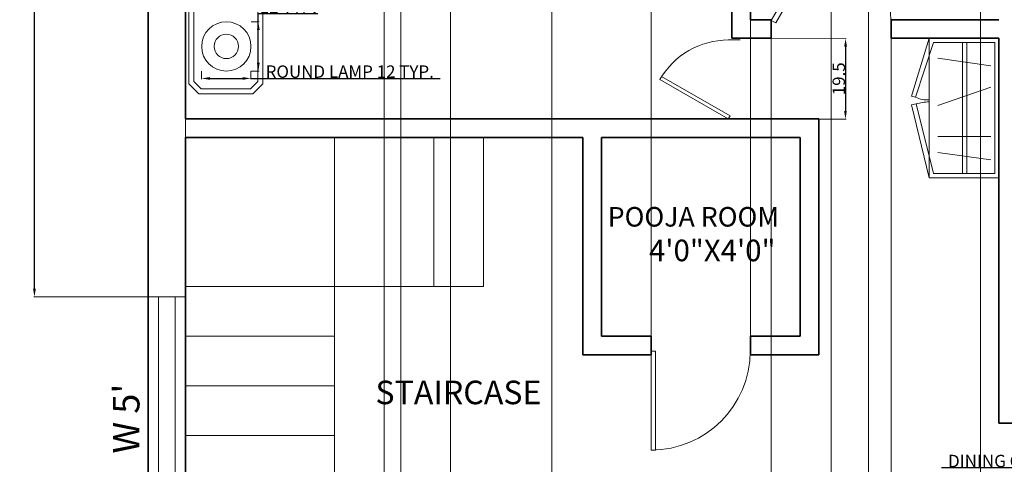
# Model space of a CAD drawing. Units: feet. Extents: x -297 to 770, y -228 to 625.
# Tile 6 of 14: x 351 to 589, y 95 to 202. Entities that reach past the tile are written whole.
import ezdxf

# ---------------------------------------------------------------- set-up
doc = ezdxf.new("R2010")
doc.units = ezdxf.units.FT
doc.header["$MEASUREMENT"] = 0
for name, color, linetype, lineweight in [('A-ANNO-DIMS', 2, 'Continuous', 18), ('A-ANNO-TEXT', 7, 'Continuous', 18), ('A-AREA-IDEN', 7, 'Continuous', 25), ('A-FLOR-STRS', 7, 'Continuous', 18), ('A-FURN', 8, 'Continuous', 18), ('A-WALL', 7, 'Continuous', 35), ('doors', 30, 'Continuous', 18), ('windows', 30, 'Continuous', 18)]:
    doc.layers.add(name, color=color, linetype=linetype, lineweight=lineweight)
doc.styles.add('Annotative', font='arial.ttf')
doc.styles.get("Standard").update_dxf_attribs({"font": 'arial.ttf'})
doc.dimstyles.get("Standard").update_dxf_attribs({"dimtxt": 3, "dimasz": 2, "dimexe": 0.18, "dimexo": 0.0625, "dimgap": 0.09, "dimtad": 1, "dimtoh": 1, "dimdec": 1, "dimzin": 0, "dimdsep": 46, "dimlunit": 3, "dimtxsty": 'Standard', "dimcen": 0, "dimclre": 256, "dimadec": 0, "dimazin": 0, "dimtfac": 1, "dimtdec": 1, "dimtofl": 0, "dimtmove": 0, "dimatfit": 3, "dimfxl": 1, "dimtolj": 1, "dimtzin": 0, "dimlwe": -1, "dimarcsym": 0})

# ---------------------------------------------------------------- blocks, each defined once
blk = doc.blocks.new('*U3')
for p, q in [((0, 0), (0, -6)), ((40, 0), (40, -6))]:
    blk.add_line(p, q)
blk.add_lwpolyline([(0, 0), (20, 34.64), (21.52, 33.77), (1.52, -0.88)], close=True)
blk.add_arc((0, 0), 40, 0, 60)
blk = doc.blocks.new('*U4')
for p, q in [((0, 0), (0, 6)), ((40, 0), (40, 6))]:
    blk.add_line(p, q)
blk.add_lwpolyline([(0, 0), (0, -40), (1.75, -40), (1.75, 0)], close=True)
blk.add_arc((0, 0), 40, 270, 0)
blk = doc.blocks.new('WIN-5FT')
for p, q in [((60, 6.5), (0, 6.5)), ((60, 2.5), (0, 2.5))]:
    blk.add_line(p, q)
blk.add_lwpolyline([(60, 0), (60, 9), (0, 9), (0, 0)], close=True)
blk = doc.blocks.new('LAMP-BEDSIDE-ROUND')
for radius in [5.95, 2.95]:
    blk.add_circle((5.95, 5.95), radius)
blk = doc.blocks.new('NIGHTSTAND')
for points in [[(17.84, 2.38), (17.84, 21.41), (15.46, 23.79), (2.38, 23.79), (0, 21.41), (0, 2.38), (2.38, 0), (15.46, 0)], [(16.65, 2.97), (16.65, 20.81), (14.87, 22.6), (2.97, 22.6), (1.19, 20.81), (1.19, 2.97), (2.97, 1.19), (14.87, 1.19)]]:
    blk.add_lwpolyline(points, close=True)
blk = doc.blocks.new('*D23')
at = {"layer": 'A-ANNO-DIMS', "color": 0, "lineweight": -2, "transparency": 16777216}
for p, q in [((620.45, 93.67), (573.78, 93.67)), ((631.66, 93.67), (622.45, 93.67))]:
    blk.add_line(p, q, dxfattribs=at)
at = {"layer": 'A-ANNO-DIMS', "transparency": 16777216}
for p, q in [((620.45, 91.75), (620.45, 93.85)), ((633.66, 91.75), (633.66, 93.85))]:
    blk.add_line(p, q, dxfattribs=at)
at = {"layer": 'A-ANNO-DIMS', "color": 0, "transparency": 16777216}
for points in [[(622.45, 94), (622.45, 93.33), (620.45, 93.67)], [(631.66, 94), (631.66, 93.33), (633.66, 93.67)]]:
    blk.add_solid(points, dxfattribs=at)
at = {"layer": 'Defpoints', "color": 0, "transparency": 16777216}
for p in [(620.45, 93.67), (620.45, 91.69), (633.66, 91.69)]:
    blk.add_point(p, dxfattribs=at)
at = {"layer": 'A-ANNO-DIMS', "color": 0, "transparency": 16777216, "insert": (596.11, 95.31), "char_height": 3, "attachment_point": 5}
blk.add_mtext('\\A1;DINING CHAIR 13 TYP.', dxfattribs=at)
blk = doc.blocks.new('*D27')
at = {"layer": 'A-ANNO-DIMS', "transparency": 16777216}
for p, q in [((395.09, 189.49), (395.09, 187.59)), ((406.99, 189.49), (406.99, 187.59))]:
    blk.add_line(p, q, dxfattribs=at)
at = {"layer": 'A-ANNO-DIMS', "color": 0, "lineweight": -2, "transparency": 16777216}
for p, q in [((397.09, 187.77), (404.99, 187.77)), ((406.99, 187.77), (452.72, 187.77))]:
    blk.add_line(p, q, dxfattribs=at)
at = {"layer": 'A-ANNO-DIMS', "color": 0, "transparency": 16777216}
for points in [[(397.09, 188.1), (397.09, 187.43), (395.09, 187.77)], [(404.99, 188.1), (404.99, 187.43), (406.99, 187.77)]]:
    blk.add_solid(points, dxfattribs=at)
at = {"layer": 'Defpoints', "color": 0, "transparency": 16777216}
for p in [(395.09, 189.55), (406.99, 189.55), (406.99, 187.77)]:
    blk.add_point(p, dxfattribs=at)
at = {"layer": 'A-ANNO-DIMS', "color": 0, "transparency": 16777216, "insert": (430.86, 189.41), "char_height": 3, "attachment_point": 5}
blk.add_mtext('\\A1;ROUND LAMP 12 TYP.', dxfattribs=at)
blk = doc.blocks.new('*D28')
at = {"layer": 'A-ANNO-DIMS', "color": 0, "lineweight": -2, "transparency": 16777216}
for p, q in [((408.77, 201.45), (408.77, 203.45)), ((408.77, 203.45), (423.18, 203.45)), ((408.77, 191.55), (408.77, 199.45))]:
    blk.add_line(p, q, dxfattribs=at)
at = {"layer": 'A-ANNO-DIMS', "transparency": 16777216}
for p, q in [((407.05, 201.45), (408.95, 201.45)), ((407.05, 189.55), (408.95, 189.55))]:
    blk.add_line(p, q, dxfattribs=at)
at = {"layer": 'A-ANNO-DIMS', "color": 0, "transparency": 16777216}
for points in [[(408.44, 199.45), (409.11, 199.45), (408.77, 201.45)], [(408.44, 191.55), (409.11, 191.55), (408.77, 189.55)]]:
    blk.add_solid(points, dxfattribs=at)
at = {"layer": 'Defpoints', "color": 0, "transparency": 16777216}
for p in [(406.99, 201.45), (408.77, 201.45), (406.99, 189.55)]:
    blk.add_point(p, dxfattribs=at)
at = {"layer": 'A-ANNO-DIMS', "color": 0, "transparency": 16777216, "insert": (416.02, 205.04), "char_height": 3, "attachment_point": 5}
blk.add_mtext('\\A1;12 TYP.', dxfattribs=at)
blk = doc.blocks.new('*D51')
at = {"layer": 'A-ANNO-DIMS', "transparency": 16777216}
for p, q in [((382.09, 306.96), (354.53, 306.96)), ((382.09, 134.96), (354.53, 134.96))]:
    blk.add_line(p, q, dxfattribs=at)
at = {"layer": 'A-ANNO-DIMS', "color": 0, "lineweight": -2, "transparency": 16777216}
blk.add_line((354.71, 136.96), (354.71, 304.96), dxfattribs=at)
at = {"layer": 'A-ANNO-DIMS', "color": 0, "transparency": 16777216}
for points in [[(354.37, 304.96), (355.04, 304.96), (354.71, 306.96)], [(354.37, 136.96), (355.04, 136.96), (354.71, 134.96)]]:
    blk.add_solid(points, dxfattribs=at)
at = {"layer": 'Defpoints', "color": 0, "transparency": 16777216}
for p in [(354.71, 306.96), (382.16, 306.96), (382.16, 134.96)]:
    blk.add_point(p, dxfattribs=at)
at = {"layer": 'A-ANNO-DIMS', "color": 0, "transparency": 16777216, "insert": (353.11, 220.96), "char_height": 3, "attachment_point": 5, "rotation": 90}
blk.add_mtext('\\A1;172', dxfattribs=at)
blk = doc.blocks.new('*D57')
at = {"layer": 'A-ANNO-DIMS', "transparency": 16777216}
for p, q in [((391.16, -163.97), (391.16, 367.22)), ((439.16, -163.97), (439.16, 367.22))]:
    blk.add_line(p, q, dxfattribs=at)
at = {"layer": 'A-ANNO-DIMS', "color": 0, "lineweight": -2, "transparency": 16777216}
blk.add_line((393.16, 367.04), (437.16, 367.04), dxfattribs=at)
at = {"layer": 'A-ANNO-DIMS', "color": 0, "transparency": 16777216}
for points in [[(393.16, 367.38), (393.16, 366.71), (391.16, 367.04)], [(437.16, 367.38), (437.16, 366.71), (439.16, 367.04)]]:
    blk.add_solid(points, dxfattribs=at)
at = {"layer": 'Defpoints', "color": 0, "transparency": 16777216}
for p in [(439.16, 367.04), (391.16, -164.04), (439.16, -164.04)]:
    blk.add_point(p, dxfattribs=at)
at = {"layer": 'A-ANNO-DIMS', "color": 0, "transparency": 16777216, "insert": (415.16, 368.66), "char_height": 3, "attachment_point": 5}
blk.add_mtext('\\A1;48', dxfattribs=at)
blk = doc.blocks.new('*D60')
at = {"layer": 'A-ANNO-DIMS', "transparency": 16777216}
for p, q in [((556.16, -144.47), (556.16, 367.22)), ((583.16, -144.47), (583.16, 367.22))]:
    blk.add_line(p, q, dxfattribs=at)
at = {"layer": 'A-ANNO-DIMS', "color": 0, "lineweight": -2, "transparency": 16777216}
blk.add_line((558.16, 367.04), (581.16, 367.04), dxfattribs=at)
at = {"layer": 'A-ANNO-DIMS', "color": 0, "transparency": 16777216}
for points in [[(558.16, 367.38), (558.16, 366.71), (556.16, 367.04)], [(581.16, 367.38), (581.16, 366.71), (583.16, 367.04)]]:
    blk.add_solid(points, dxfattribs=at)
at = {"layer": 'Defpoints', "color": 0, "transparency": 16777216}
for p in [(583.16, 367.04), (556.16, -144.54), (583.16, -144.54)]:
    blk.add_point(p, dxfattribs=at)
at = {"layer": 'A-ANNO-DIMS', "color": 0, "transparency": 16777216, "insert": (569.66, 368.64), "char_height": 3, "attachment_point": 5}
blk.add_mtext('\\A1;27', dxfattribs=at)
blk = doc.blocks.new('*D66')
at = {"layer": 'A-ANNO-DIMS', "transparency": 16777216}
for p, q in [((503.66, 125.53), (503.66, 367.22)), ((527.66, 125.53), (527.66, 367.22))]:
    blk.add_line(p, q, dxfattribs=at)
at = {"layer": 'A-ANNO-DIMS', "color": 0, "lineweight": -2, "transparency": 16777216}
blk.add_line((505.66, 367.04), (525.66, 367.04), dxfattribs=at)
at = {"layer": 'A-ANNO-DIMS', "color": 0, "transparency": 16777216}
for points in [[(505.66, 367.38), (505.66, 366.71), (503.66, 367.04)], [(525.66, 367.38), (525.66, 366.71), (527.66, 367.04)]]:
    blk.add_solid(points, dxfattribs=at)
at = {"layer": 'Defpoints', "color": 0, "transparency": 16777216}
for p in [(527.66, 367.04), (503.66, 125.46), (527.66, 125.46)]:
    blk.add_point(p, dxfattribs=at)
at = {"layer": 'A-ANNO-DIMS', "color": 0, "transparency": 16777216, "insert": (515.66, 368.64), "char_height": 3, "attachment_point": 5}
blk.add_mtext('\\A1;24', dxfattribs=at)
blk = doc.blocks.new('*D67')
at = {"layer": 'A-ANNO-DIMS', "transparency": 16777216}
for p, q in [((532.66, 197.4), (532.66, -227.67)), ((561.66, 197.4), (561.66, -227.67))]:
    blk.add_line(p, q, dxfattribs=at)
at = {"layer": 'A-ANNO-DIMS', "color": 0, "lineweight": -2, "transparency": 16777216}
blk.add_line((534.66, -227.49), (559.66, -227.49), dxfattribs=at)
at = {"layer": 'A-ANNO-DIMS', "color": 0, "transparency": 16777216}
for points in [[(534.66, -227.15), (534.66, -227.82), (532.66, -227.49)], [(559.66, -227.15), (559.66, -227.82), (561.66, -227.49)]]:
    blk.add_solid(points, dxfattribs=at)
at = {"layer": 'Defpoints', "color": 0, "transparency": 16777216}
for p in [(532.66, 197.46), (561.66, 197.46), (561.66, -227.49)]:
    blk.add_point(p, dxfattribs=at)
at = {"layer": 'A-ANNO-DIMS', "color": 0, "transparency": 16777216, "insert": (547.16, -225.87), "char_height": 3, "attachment_point": 5}
blk.add_mtext('\\A1;29', dxfattribs=at)
blk = doc.blocks.new('*D71')
at = {"layer": 'A-ANNO-DIMS', "transparency": 16777216}
for p, q in [((523.22, 197.46), (550.79, 197.42)), ((523.19, 177.96), (550.76, 177.92))]:
    blk.add_line(p, q, dxfattribs=at)
at = {"layer": 'A-ANNO-DIMS', "color": 0, "lineweight": -2, "transparency": 16777216}
blk.add_line((550.6, 195.42), (550.58, 179.92), dxfattribs=at)
at = {"layer": 'A-ANNO-DIMS', "color": 0, "transparency": 16777216}
for points in [[(550.27, 195.42), (550.94, 195.42), (550.61, 197.42)], [(550.25, 179.92), (550.91, 179.92), (550.58, 177.92)]]:
    blk.add_solid(points, dxfattribs=at)
at = {"layer": 'Defpoints', "color": 0, "transparency": 16777216}
for p in [(523.16, 197.46), (523.13, 177.96), (550.58, 177.92)]:
    blk.add_point(p, dxfattribs=at)
at = {"layer": 'A-ANNO-DIMS', "color": 0, "transparency": 16777216, "insert": (548.97, 187.68), "char_height": 3, "attachment_point": 5, "rotation": 89.9165}
blk.add_mtext('\\A1;19.5', dxfattribs=at)
blk = doc.blocks.new('*D72')
at = {"layer": 'A-ANNO-DIMS', "transparency": 16777216}
for p, q in [((479.66, 49.03), (479.66, 367.22)), ((547.16, 49.03), (547.16, 367.22))]:
    blk.add_line(p, q, dxfattribs=at)
at = {"layer": 'A-ANNO-DIMS', "color": 0, "lineweight": -2, "transparency": 16777216}
blk.add_line((481.66, 367.04), (545.16, 367.04), dxfattribs=at)
at = {"layer": 'A-ANNO-DIMS', "color": 0, "transparency": 16777216}
for points in [[(481.66, 367.38), (481.66, 366.71), (479.66, 367.04)], [(545.16, 367.38), (545.16, 366.71), (547.16, 367.04)]]:
    blk.add_solid(points, dxfattribs=at)
at = {"layer": 'Defpoints', "color": 0, "transparency": 16777216}
for p in [(547.16, 367.04), (479.66, 48.96), (547.16, 48.96)]:
    blk.add_point(p, dxfattribs=at)
at = {"layer": 'A-ANNO-DIMS', "color": 0, "transparency": 16777216, "insert": (513.41, 368.66), "char_height": 3, "attachment_point": 5}
blk.add_mtext('\\A1;67.5', dxfattribs=at)
blk = doc.blocks.new('*D76')
at = {"layer": 'A-ANNO-DIMS', "transparency": 16777216}
for p, q in [((443.16, 89.53), (443.16, 367.22)), ((455.16, 89.53), (455.16, 367.22))]:
    blk.add_line(p, q, dxfattribs=at)
at = {"layer": 'A-ANNO-DIMS', "color": 0, "lineweight": -2, "transparency": 16777216}
blk.add_line((445.16, 367.04), (453.16, 367.04), dxfattribs=at)
at = {"layer": 'A-ANNO-DIMS', "color": 0, "transparency": 16777216}
for points in [[(445.16, 367.38), (445.16, 366.71), (443.16, 367.04)], [(453.16, 367.38), (453.16, 366.71), (455.16, 367.04)]]:
    blk.add_solid(points, dxfattribs=at)
at = {"layer": 'Defpoints', "color": 0, "transparency": 16777216}
for p in [(455.16, 367.04), (443.16, 89.46), (455.16, 89.46)]:
    blk.add_point(p, dxfattribs=at)
at = {"layer": 'A-ANNO-DIMS', "color": 0, "transparency": 16777216, "insert": (449.16, 368.64), "char_height": 3, "attachment_point": 5}
blk.add_mtext('\\A1;12', dxfattribs=at)

msp = doc.modelspace()

# ---------------------------------------------------------------- linework, layer by layer
at = {"layer": 'A-FLOR-STRS'}
for p, q in [((427.155, 89.463), (427.155, 173.463)), ((439.155, 137.463), (439.155, 173.463)), ((451.155, 137.463), (451.155, 173.463)), ((463.155, 137.463), (463.155, 173.463)), ((463.155, 137.463), (391.155, 137.463)), ((427.155, 125.463), (391.155, 125.463)), ((427.155, 113.463), (391.155, 113.463)), ((427.155, 101.463), (391.155, 101.463))]:
    msp.add_line(p, q, dxfattribs=at)
at = {"layer": 'A-FURN'}
for p, q in [((566.554, 183.497), (570.809, 197.463)), ((570.809, 197.463), (566.554, 183.497)), ((587.655, 197.463), (570.809, 197.463)), ((570.809, 197.463), (570.809, 163.771)), ((587.655, 163.771), (587.655, 197.463)), ((567.533, 183.209), (571.82, 196.452)), ((586.645, 196.452), (571.82, 196.452)), ((578.877, 164.773), (578.877, 196.46)), ((579.888, 164.773), (579.888, 196.46)), ((586.645, 164.781), (586.645, 196.452)), ((572.888, 192.658), (585.729, 190.814)), ((572.888, 181.193), (585.729, 185.687)), ((566.554, 183.497), (567.533, 183.209)), ((566.554, 181.423), (567.648, 181.654)), ((570.809, 163.771), (566.554, 181.423)), ((567.648, 181.654), (571.82, 164.781)), ((572.888, 173.761), (585.729, 173.761)), ((585.729, 168.057), (572.888, 169.901)), ((571.82, 164.781), (586.645, 164.781)), ((570.809, 163.771), (587.655, 163.771))]:
    msp.add_line(p, q, dxfattribs=at)
for centre, radius, start, end in [((570.328, 188.91), 6.349, 243.88148, 273.88148), ((571.82, 164.781), 17.38, 93.39424, 103.88926)]:
    msp.add_arc(centre, radius, start, end, dxfattribs=at)
at = {"layer": 'A-WALL'}
for p, q in [((523.155, 197.463), (523.155, 297.963)), ((527.655, 201.963), (527.655, 297.963)), ((532.655, 201.963), (527.655, 201.963)), ((532.655, 201.963), (532.655, 197.463)), ((587.655, 201.963), (561.655, 201.963)), ((561.655, 201.963), (561.655, 197.463)), ((532.655, 197.463), (523.155, 197.463)), ((587.655, 197.463), (561.655, 197.463)), ((587.655, 197.463), (587.655, 104.463)), ((544.155, 177.963), (391.155, 177.963)), ((544.155, 177.963), (544.155, 120.963)), ((487.155, 173.463), (391.155, 173.463)), ((487.155, 173.463), (487.155, 120.963)), ((539.655, 173.463), (491.655, 173.463)), ((491.655, 173.463), (491.655, 125.463)), ((539.655, 173.463), (539.655, 125.463)), ((491.655, 125.463), (503.655, 125.463)), ((503.655, 125.463), (503.655, 120.963)), ((527.655, 125.463), (527.655, 120.963)), ((527.655, 125.463), (539.655, 125.463)), ((487.155, 120.963), (503.655, 120.963)), ((527.655, 120.963), (544.155, 120.963)), ((587.655, 104.463), (612.155, 104.463))]:
    msp.add_line(p, q, dxfattribs=at)
for points in [[(685.155, 306.963), (382.155, 306.963), (382.155, -173.037), (556.155, -173.037)], [(523.155, 297.963), (391.155, 297.963), (391.155, 177.963)], [(391.155, 173.463), (391.155, -11.037)]]:
    msp.add_lwpolyline(points, dxfattribs=at)

# ---------------------------------------------------------------- block references
at = {"layer": 'A-FURN'}
for name, p in [('NIGHTSTAND', (392, 184.081)), ('LAMP-BEDSIDE-ROUND', (395.094, 189.552))]:
    msp.add_blockref(name, p, dxfattribs=at)
at = {"layer": 'doors'}
for name, p, xscale, yscale, zscale in [('*U3', (532.655, 201.799), 0.7226421799388985, 0.7226421799388985, 0.7226421799388985), ('*U4', (503.655, 121.878), 0.598122456182507, 0.598122456182507, 0.598122456182507)]:
    msp.add_blockref(name, p, dxfattribs=dict(at, xscale=xscale, yscale=yscale, zscale=zscale))
at = {"layer": 'doors', "xscale": 0.4772717043500036, "yscale": 0.4772717043500036, "zscale": 0.4772717043500036, "rotation": 90}
msp.add_blockref('*U3', (522.292, 177.963), dxfattribs=at)
at = {"layer": 'windows', "rotation": 90.00000000000003}
msp.add_blockref('WIN-5FT', (391.155, 74.963), dxfattribs=at)

# ---------------------------------------------------------------- texts
at = {"layer": 'A-ANNO-TEXT', "style": 'Annotative'}
msp.add_text("W 5'", height=6.4048, rotation=90, dxfattribs=at).set_placement((380.073, 97.115))
at = {"layer": 'A-AREA-IDEN', "style": 'Annotative'}
for s, height, p in [('POOJA ROOM', 4.7287, (493.155, 151.963)), ('4\'0"X4\'0"', 5.2107, (503.14, 143.592)), ('STAIRCASE', 5.696, (437.053, 109.038))]:
    msp.add_text(s, height=height, dxfattribs=at).set_placement(p)

# ---------------------------------------------------------------- dimensions: what is measured, and where the dimension line sits
at = {"layer": 'A-ANNO-DIMS'}
for base, p1, p2, override, picture, middle in [((439.155, 367.042), (391.155, -164.037), (439.155, -164.037), {"dimdec": 0, "dimlfac": 1, "dimrnd": 0, "dimzin": 0, "dimdsep": 46, "dimlunit": 2}, '*D57', (415.155, 368.664)), ((455.155, 367.042), (443.155, 89.463), (455.155, 89.463), {"dimdec": 0, "dimlfac": 1, "dimrnd": 0, "dimzin": 0, "dimdsep": 46, "dimlunit": 2}, '*D76', (449.155, 368.638)), ((547.155, 367.042), (479.655, 48.963), (547.155, 48.963), {"dimdec": 1, "dimlfac": 1, "dimrnd": 0, "dimzin": 0, "dimdsep": 46, "dimlunit": 2}, '*D72', (513.405, 368.664)), ((527.655, 367.042), (503.655, 125.463), (527.655, 125.463), {"dimdec": 0, "dimlfac": 1, "dimrnd": 0, "dimzin": 0, "dimdsep": 46, "dimlunit": 2}, '*D66', (515.655, 368.638)), ((583.155, 367.042), (556.155, -144.537), (583.155, -144.537), {"dimdec": 0, "dimlfac": 1, "dimrnd": 0, "dimzin": 0, "dimdsep": 46, "dimlunit": 2}, '*D60', (569.655, 368.638)), ((561.655, -227.487), (532.655, 197.463), (561.655, 197.463), {"dimdec": 0, "dimlfac": 1, "dimrnd": 0, "dimzin": 0, "dimdsep": 46, "dimlunit": 2}, '*D67', (547.155, -225.866))]:
    dim = msp.add_linear_dim(base=base, p1=p1, p2=p2, dimstyle='Standard', override=override, dxfattribs=at)
    dim.commit()
    dim.dimension.update_dxf_attribs({"geometry": picture, "text_midpoint": middle})
for base, p1, p2, angle, override, picture, middle in [((354.705, 306.963), (382.155, 134.963), (382.155, 306.963), 90, {"dimdec": 0, "dimlfac": 1, "dimrnd": 0, "dimzin": 0, "dimdsep": 46, "dimlunit": 2}, '*D51', (353.109, 220.963)), ((550.577, 177.923), (523.155, 197.463), (523.127, 177.963), 269.91654, {"dimdec": 1, "dimlfac": 1, "dimrnd": 0, "dimzin": 0, "dimdsep": 46, "dimlunit": 2}, '*D71', (548.969, 187.675))]:
    dim = msp.add_linear_dim(base=base, p1=p1, p2=p2, angle=angle, dimstyle='Standard', override=override, dxfattribs=at)
    dim.commit()
    dim.dimension.update_dxf_attribs({"geometry": picture, "text_midpoint": middle})
for base, p1, p2, angle, text, picture, middle in [((408.772, 201.447), (406.988, 189.552), (406.988, 201.447), 90, '<> TYP.', '*D28', (416.023, 205.044)), ((620.45, 93.666), (633.656, 91.685), (620.45, 91.685), 180, 'DINING CHAIR <> TYP.', '*D23', (596.115, 95.309))]:
    dim = msp.add_linear_dim(base=base, p1=p1, p2=p2, angle=angle, text=text, dimstyle='Standard', override={"dimdec": 0, "dimlfac": 1, "dimrnd": 0, "dimzin": 0, "dimdsep": 46, "dimlunit": 2}, dxfattribs=at)
    dim.commit()
    dim.dimension.update_dxf_attribs({"geometry": picture, "text_midpoint": middle})
dim = msp.add_linear_dim(base=(406.988, 187.768), p1=(395.094, 189.552), p2=(406.988, 189.552), text='ROUND LAMP <> TYP.', dimstyle='Standard', override={"dimdec": 0, "dimlfac": 1, "dimrnd": 0, "dimzin": 0, "dimdsep": 46, "dimlunit": 2}, dxfattribs=at)
dim.commit()
dim.dimension.update_dxf_attribs({"geometry": '*D27', "text_midpoint": (430.856, 189.41)})

doc.saveas('drawing.dxf')
